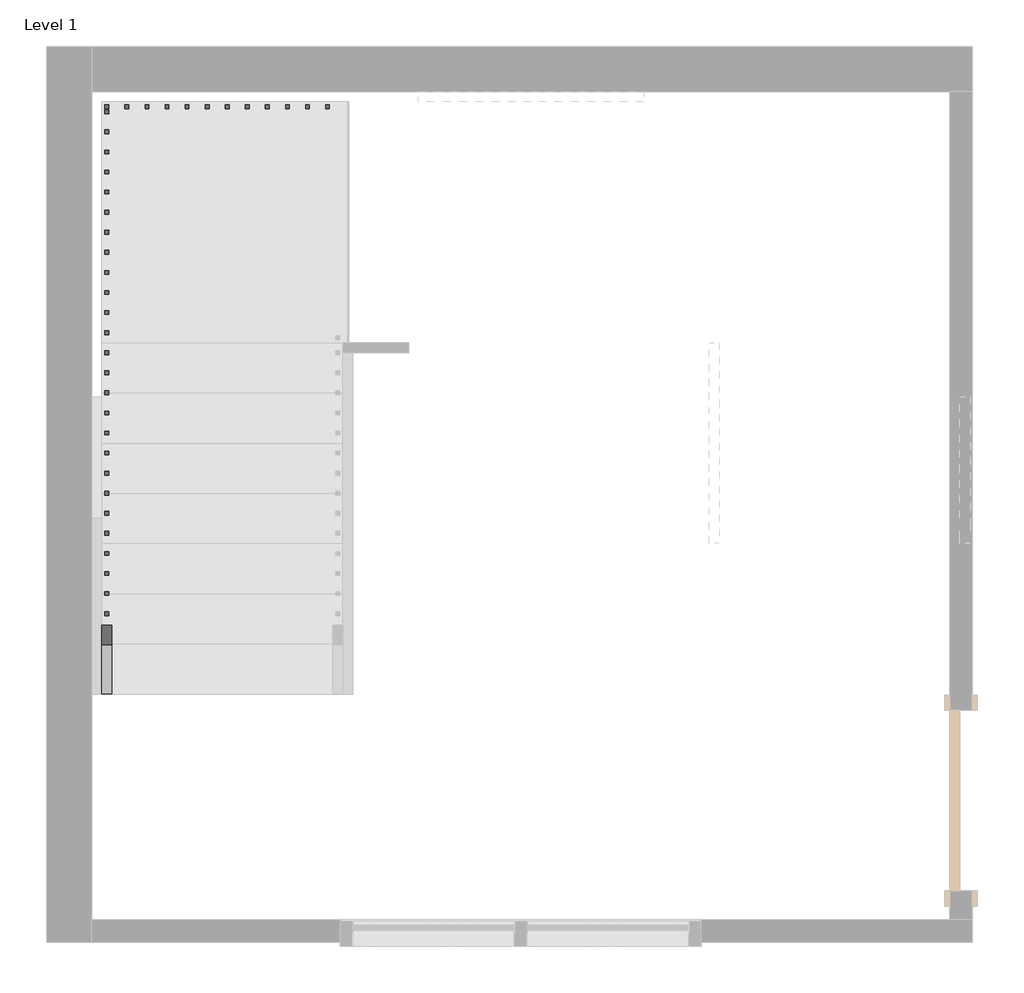
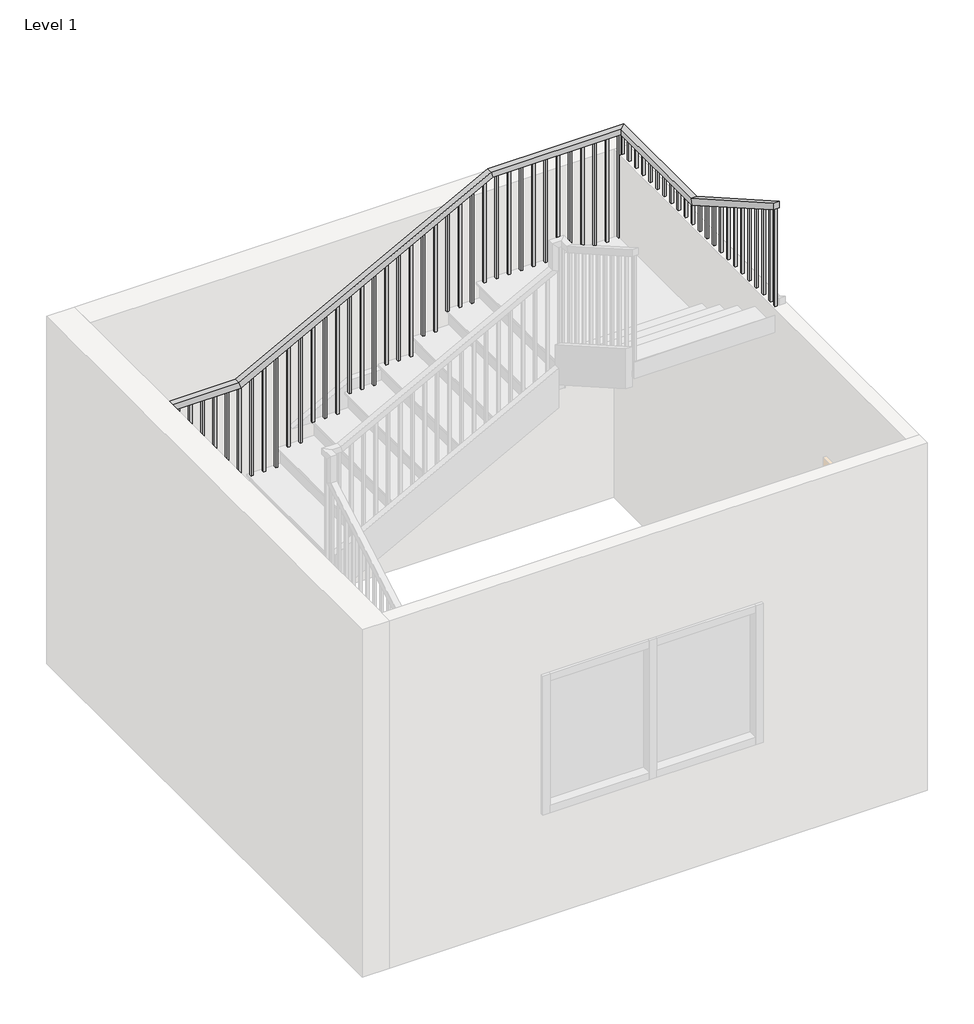
# One storey, part 5 of 9: 1 railing.
"""IFC4 building model written with IfcOpenShell, lengths in millimetres."""

from ifc_helpers import new_model, si_unit, frame, origin, place, context, project, spatial, polyline, outline, extrude, faceted_brep, element, save

model = new_model("IFC4")

# Units and contexts
model_context = context("Model", 3, world=origin())
ifc_project = project(units=[si_unit("LENGTHUNIT", "METRE", prefix="MILLI")], contexts=[model_context])

# Site, building, storey
site = spatial("IfcSite", under=ifc_project)
building = spatial("IfcBuilding", under=site)
storey = spatial("IfcBuildingStorey", under=building, Name="Level 1", Elevation=0.0)

# Railing
placement = place(None, origin())
element("IfcRailing", 1, ObjectType="Handrail - Rectangular", at=placement, inside=storey, context=model_context, shape_type="SolidModel", body=[
    faceted_brep([(-63763.8636189, 6754.3199577, 1059.5428571), (-63763.8636189, 6754.3199577, 1001.0339009), (-63713.0636189, 6754.3199577, 1001.0339009), (-63713.0636189, 6754.3199577, 1059.5428571), (-63763.8636189, 8699.113291, 2170.8533333), (-63763.8636189, 8712.6039644, 2120.0533333), (-63713.0636189, 8712.6039644, 2120.0533333), (-63713.0636189, 8699.113291, 2170.8533333), (-63763.8636189, 9751.5199577, 2170.8533333), (-63763.8636189, 9751.5199577, 2120.0533333), (-63713.0636189, 9700.7199577, 2120.0533333), (-63713.0636189, 9700.7199577, 2170.8533333), (-62638.0993332, 9751.5199577, 2170.8533333), (-62625.3993332, 9751.5199577, 2120.0533333), (-62625.3993332, 9700.7199577, 2120.0533333), (-62638.0993332, 9700.7199577, 2170.8533333), (-60546.2279046, 9751.5199577, 3286.5180952), (-60533.5279046, 9751.5199577, 3235.7180952), (-60533.5279046, 9700.7199577, 3235.7180952), (-60546.2279046, 9700.7199577, 3286.5180952), (-59420.4636189, 9751.5199577, 3286.5180952), (-59420.4636189, 9751.5199577, 3235.7180952), (-59471.2636189, 9700.7199577, 3235.7180952), (-59471.2636189, 9700.7199577, 3286.5180952), (-59420.4636189, 8699.113291, 3286.5180952), (-59420.4636189, 8685.6226176, 3235.7180952), (-59471.2636189, 8685.6226176, 3235.7180952), (-59471.2636189, 8699.113291, 3286.5180952), (-59420.4636189, 7516.3199577, 3962.4), (-59471.2636189, 7516.3199577, 3962.4), (-59471.2636189, 7516.3199577, 3903.8910438), (-59420.4636189, 7516.3199577, 3903.8910438)], [[[0, 1, 2, 3]], [[1, 0, 4, 5]], [[2, 1, 5, 6]], [[3, 2, 6, 7]], [[0, 3, 7, 4]], [[5, 4, 8, 9]], [[6, 5, 9, 10]], [[7, 6, 10, 11]], [[4, 7, 11, 8]], [[9, 8, 12, 13]], [[10, 9, 13, 14]], [[11, 10, 14, 15]], [[8, 11, 15, 12]], [[13, 12, 16, 17]], [[14, 13, 17, 18]], [[15, 14, 18, 19]], [[12, 15, 19, 16]], [[17, 16, 20, 21]], [[18, 17, 21, 22]], [[19, 18, 22, 23]], [[16, 19, 23, 20]], [[21, 20, 24, 25]], [[22, 21, 25, 26]], [[23, 22, 26, 27]], [[20, 23, 27, 24]], [[28, 29, 30, 31]], [[25, 24, 28, 31]], [[26, 25, 31, 30]], [[27, 26, 30, 29]], [[24, 27, 29, 28]]]),
    extrude(outline(polyline([(7602.0449577, 3854.9053295), (7602.0449577, 2902.8571429), (7582.9949577, 2902.8571429), (7582.9949577, 3865.7910438), (7602.0449577, 3854.9053295)])), frame((-59455.3886189, 0.0, 0.0), z_axis=(1.0, 0.0, 0.0), x_axis=(0.0, 1.0, 0.0)), (0.0, 0.0, 1.0), 19.05),
    extrude(outline(polyline([(7703.6449577, 3796.8481866), (7703.6449577, 2902.8571429), (7684.5949577, 2902.8571429), (7684.5949577, 3807.7339009), (7703.6449577, 3796.8481866)])), frame((-59455.3886189, 0.0, 0.0), z_axis=(1.0, 0.0, 0.0), x_axis=(0.0, 1.0, 0.0)), (0.0, 0.0, 1.0), 19.05),
    extrude(outline(polyline([(7805.2449577, 3738.7910438), (7805.2449577, 2757.7142857), (7786.1949577, 2757.7142857), (7786.1949577, 3749.6767581), (7805.2449577, 3738.7910438)])), frame((-59455.3886189, 0.0, 0.0), z_axis=(1.0, 0.0, 0.0), x_axis=(0.0, 1.0, 0.0)), (0.0, 0.0, 1.0), 19.05),
    extrude(outline(polyline([(7906.8449577, 3680.7339009), (7906.8449577, 2757.7142857), (7887.7949577, 2757.7142857), (7887.7949577, 3691.6196152), (7906.8449577, 3680.7339009)])), frame((-59455.3886189, 0.0, 0.0), z_axis=(1.0, 0.0, 0.0), x_axis=(0.0, 1.0, 0.0)), (0.0, 0.0, 1.0), 19.05),
    extrude(outline(polyline([(8008.4449577, 3622.6767581), (8008.4449577, 2757.7142857), (7989.3949577, 2757.7142857), (7989.3949577, 3633.5624723), (8008.4449577, 3622.6767581)])), frame((-59455.3886189, 0.0, 0.0), z_axis=(1.0, 0.0, 0.0), x_axis=(0.0, 1.0, 0.0)), (0.0, 0.0, 1.0), 19.05),
    extrude(outline(polyline([(8110.0449577, 3564.6196152), (8110.0449577, 2612.5714286), (8090.9949577, 2612.5714286), (8090.9949577, 3575.5053295), (8110.0449577, 3564.6196152)])), frame((-59455.3886189, 0.0, 0.0), z_axis=(1.0, 0.0, 0.0), x_axis=(0.0, 1.0, 0.0)), (0.0, 0.0, 1.0), 19.05),
    extrude(outline(polyline([(8211.6449577, 3506.5624723), (8211.6449577, 2612.5714286), (8192.5949577, 2612.5714286), (8192.5949577, 3517.4481866), (8211.6449577, 3506.5624723)])), frame((-59455.3886189, 0.0, 0.0), z_axis=(1.0, 0.0, 0.0), x_axis=(0.0, 1.0, 0.0)), (0.0, 0.0, 1.0), 19.05),
    extrude(outline(polyline([(8313.2449577, 3448.5053295), (8313.2449577, 2467.4285714), (8294.1949577, 2467.4285714), (8294.1949577, 3459.3910438), (8313.2449577, 3448.5053295)])), frame((-59455.3886189, 0.0, 0.0), z_axis=(1.0, 0.0, 0.0), x_axis=(0.0, 1.0, 0.0)), (0.0, 0.0, 1.0), 19.05),
    extrude(outline(polyline([(8414.8449577, 3390.4481866), (8414.8449577, 2467.4285714), (8395.7949577, 2467.4285714), (8395.7949577, 3401.3339009), (8414.8449577, 3390.4481866)])), frame((-59455.3886189, 0.0, 0.0), z_axis=(1.0, 0.0, 0.0), x_axis=(0.0, 1.0, 0.0)), (0.0, 0.0, 1.0), 19.05),
    extrude(outline(polyline([(8516.4449577, 3332.3910438), (8516.4449577, 2467.4285714), (8497.3949577, 2467.4285714), (8497.3949577, 3343.2767581), (8516.4449577, 3332.3910438)])), frame((-59455.3886189, 0.0, 0.0), z_axis=(1.0, 0.0, 0.0), x_axis=(0.0, 1.0, 0.0)), (0.0, 0.0, 1.0), 19.05),
    extrude(outline(polyline([(8618.0449577, 3274.3339009), (8618.0449577, 2322.2857143), (8598.9949577, 2322.2857143), (8598.9949577, 3285.2196152), (8618.0449577, 3274.3339009)])), frame((-59455.3886189, 0.0, 0.0), z_axis=(1.0, 0.0, 0.0), x_axis=(0.0, 1.0, 0.0)), (0.0, 0.0, 1.0), 19.05),
    extrude(outline(polyline([(-59436.3386189, 8719.6449577), (-59436.3386189, 8700.5949577), (-59455.3886189, 8700.5949577), (-59455.3886189, 8719.6449577), (-59436.3386189, 8719.6449577)])), frame((0.0, 0.0, 2322.2857143), z_axis=(0.0, 0.0, 1.0), x_axis=(1.0, 0.0, 0.0)), (0.0, 0.0, 1.0), 913.432381),
    extrude(outline(polyline([(-59436.3386189, 8821.2449577), (-59436.3386189, 8802.1949577), (-59455.3886189, 8802.1949577), (-59455.3886189, 8821.2449577), (-59436.3386189, 8821.2449577)])), frame((0.0, 0.0, 2322.2857143), z_axis=(0.0, 0.0, 1.0), x_axis=(1.0, 0.0, 0.0)), (0.0, 0.0, 1.0), 913.432381),
    extrude(outline(polyline([(-59436.3386189, 8922.8449577), (-59436.3386189, 8903.7949577), (-59455.3886189, 8903.7949577), (-59455.3886189, 8922.8449577), (-59436.3386189, 8922.8449577)])), frame((0.0, 0.0, 2322.2857143), z_axis=(0.0, 0.0, 1.0), x_axis=(1.0, 0.0, 0.0)), (0.0, 0.0, 1.0), 913.432381),
    extrude(outline(polyline([(-59436.3386189, 9024.4449577), (-59436.3386189, 9005.3949577), (-59455.3886189, 9005.3949577), (-59455.3886189, 9024.4449577), (-59436.3386189, 9024.4449577)])), frame((0.0, 0.0, 2322.2857143), z_axis=(0.0, 0.0, 1.0), x_axis=(1.0, 0.0, 0.0)), (0.0, 0.0, 1.0), 913.432381),
    extrude(outline(polyline([(-59436.3386189, 9126.0449577), (-59436.3386189, 9106.9949577), (-59455.3886189, 9106.9949577), (-59455.3886189, 9126.0449577), (-59436.3386189, 9126.0449577)])), frame((0.0, 0.0, 2322.2857143), z_axis=(0.0, 0.0, 1.0), x_axis=(1.0, 0.0, 0.0)), (0.0, 0.0, 1.0), 913.432381),
    extrude(outline(polyline([(-59436.3386189, 9227.6449577), (-59436.3386189, 9208.5949577), (-59455.3886189, 9208.5949577), (-59455.3886189, 9227.6449577), (-59436.3386189, 9227.6449577)])), frame((0.0, 0.0, 2322.2857143), z_axis=(0.0, 0.0, 1.0), x_axis=(1.0, 0.0, 0.0)), (0.0, 0.0, 1.0), 913.432381),
    extrude(outline(polyline([(-59436.3386189, 9329.2449577), (-59436.3386189, 9310.1949577), (-59455.3886189, 9310.1949577), (-59455.3886189, 9329.2449577), (-59436.3386189, 9329.2449577)])), frame((0.0, 0.0, 2322.2857143), z_axis=(0.0, 0.0, 1.0), x_axis=(1.0, 0.0, 0.0)), (0.0, 0.0, 1.0), 913.432381),
    extrude(outline(polyline([(-59436.3386189, 9430.8449577), (-59436.3386189, 9411.7949577), (-59455.3886189, 9411.7949577), (-59455.3886189, 9430.8449577), (-59436.3386189, 9430.8449577)])), frame((0.0, 0.0, 2322.2857143), z_axis=(0.0, 0.0, 1.0), x_axis=(1.0, 0.0, 0.0)), (0.0, 0.0, 1.0), 913.432381),
    extrude(outline(polyline([(-59436.3386189, 9532.4449577), (-59436.3386189, 9513.3949577), (-59455.3886189, 9513.3949577), (-59455.3886189, 9532.4449577), (-59436.3386189, 9532.4449577)])), frame((0.0, 0.0, 2322.2857143), z_axis=(0.0, 0.0, 1.0), x_axis=(1.0, 0.0, 0.0)), (0.0, 0.0, 1.0), 913.432381),
    extrude(outline(polyline([(-59436.3386189, 9634.0449577), (-59436.3386189, 9614.9949577), (-59455.3886189, 9614.9949577), (-59455.3886189, 9634.0449577), (-59436.3386189, 9634.0449577)])), frame((0.0, 0.0, 2322.2857143), z_axis=(0.0, 0.0, 1.0), x_axis=(1.0, 0.0, 0.0)), (0.0, 0.0, 1.0), 913.432381),
    extrude(outline(polyline([(-59480.7886189, 9735.6449577), (-59461.7386189, 9735.6449577), (-59461.7386189, 9716.5949577), (-59480.7886189, 9716.5949577), (-59480.7886189, 9735.6449577)])), frame((0.0, 0.0, 2322.2857143), z_axis=(0.0, 0.0, 1.0), x_axis=(1.0, 0.0, 0.0)), (0.0, 0.0, 1.0), 913.432381),
    extrude(outline(polyline([(-59582.3886189, 9735.6449577), (-59563.3386189, 9735.6449577), (-59563.3386189, 9716.5949577), (-59582.3886189, 9716.5949577), (-59582.3886189, 9735.6449577)])), frame((0.0, 0.0, 2322.2857143), z_axis=(0.0, 0.0, 1.0), x_axis=(1.0, 0.0, 0.0)), (0.0, 0.0, 1.0), 913.432381),
    extrude(outline(polyline([(-59683.9886189, 9735.6449577), (-59664.9386189, 9735.6449577), (-59664.9386189, 9716.5949577), (-59683.9886189, 9716.5949577), (-59683.9886189, 9735.6449577)])), frame((0.0, 0.0, 2322.2857143), z_axis=(0.0, 0.0, 1.0), x_axis=(1.0, 0.0, 0.0)), (0.0, 0.0, 1.0), 913.432381),
    extrude(outline(polyline([(-59785.5886189, 9735.6449577), (-59766.5386189, 9735.6449577), (-59766.5386189, 9716.5949577), (-59785.5886189, 9716.5949577), (-59785.5886189, 9735.6449577)])), frame((0.0, 0.0, 2322.2857143), z_axis=(0.0, 0.0, 1.0), x_axis=(1.0, 0.0, 0.0)), (0.0, 0.0, 1.0), 913.432381),
    extrude(outline(polyline([(-59887.1886189, 9735.6449577), (-59868.1386189, 9735.6449577), (-59868.1386189, 9716.5949577), (-59887.1886189, 9716.5949577), (-59887.1886189, 9735.6449577)])), frame((0.0, 0.0, 2322.2857143), z_axis=(0.0, 0.0, 1.0), x_axis=(1.0, 0.0, 0.0)), (0.0, 0.0, 1.0), 913.432381),
    extrude(outline(polyline([(-59988.7886189, 9735.6449577), (-59969.7386189, 9735.6449577), (-59969.7386189, 9716.5949577), (-59988.7886189, 9716.5949577), (-59988.7886189, 9735.6449577)])), frame((0.0, 0.0, 2322.2857143), z_axis=(0.0, 0.0, 1.0), x_axis=(1.0, 0.0, 0.0)), (0.0, 0.0, 1.0), 913.432381),
    extrude(outline(polyline([(-60090.3886189, 9735.6449577), (-60071.3386189, 9735.6449577), (-60071.3386189, 9716.5949577), (-60090.3886189, 9716.5949577), (-60090.3886189, 9735.6449577)])), frame((0.0, 0.0, 2322.2857143), z_axis=(0.0, 0.0, 1.0), x_axis=(1.0, 0.0, 0.0)), (0.0, 0.0, 1.0), 913.432381),
    extrude(outline(polyline([(-60191.9886189, 9735.6449577), (-60172.9386189, 9735.6449577), (-60172.9386189, 9716.5949577), (-60191.9886189, 9716.5949577), (-60191.9886189, 9735.6449577)])), frame((0.0, 0.0, 2322.2857143), z_axis=(0.0, 0.0, 1.0), x_axis=(1.0, 0.0, 0.0)), (0.0, 0.0, 1.0), 913.432381),
    extrude(outline(polyline([(-60293.5886189, 9735.6449577), (-60274.5386189, 9735.6449577), (-60274.5386189, 9716.5949577), (-60293.5886189, 9716.5949577), (-60293.5886189, 9735.6449577)])), frame((0.0, 0.0, 2322.2857143), z_axis=(0.0, 0.0, 1.0), x_axis=(1.0, 0.0, 0.0)), (0.0, 0.0, 1.0), 913.432381),
    extrude(outline(polyline([(-60395.1886189, 9735.6449577), (-60376.1386189, 9735.6449577), (-60376.1386189, 9716.5949577), (-60395.1886189, 9716.5949577), (-60395.1886189, 9735.6449577)])), frame((0.0, 0.0, 2322.2857143), z_axis=(0.0, 0.0, 1.0), x_axis=(1.0, 0.0, 0.0)), (0.0, 0.0, 1.0), 913.432381),
    extrude(outline(polyline([(-60496.7886189, 9735.6449577), (-60477.7386189, 9735.6449577), (-60477.7386189, 9716.5949577), (-60496.7886189, 9716.5949577), (-60496.7886189, 9735.6449577)])), frame((0.0, 0.0, 2322.2857143), z_axis=(0.0, 0.0, 1.0), x_axis=(1.0, 0.0, 0.0)), (0.0, 0.0, 1.0), 913.432381),
    extrude(outline(polyline([(3201.1257143, -60598.3886189), (2322.2857143, -60598.3886189), (2322.2857143, -60579.3386189), (3211.2857143, -60579.3386189), (3201.1257143, -60598.3886189)])), frame((0.0, 9716.5949577, 0.0), z_axis=(0.0, 1.0, 0.0), x_axis=(0.0, 0.0, 1.0)), (0.0, 0.0, 1.0), 19.05),
    extrude(outline(polyline([(3146.9390476, -60699.9886189), (2177.1428571, -60699.9886189), (2177.1428571, -60680.9386189), (3157.0990476, -60680.9386189), (3146.9390476, -60699.9886189)])), frame((0.0, 9716.5949577, 0.0), z_axis=(0.0, 1.0, 0.0), x_axis=(0.0, 0.0, 1.0)), (0.0, 0.0, 1.0), 19.05),
    extrude(outline(polyline([(3092.752381, -60801.5886189), (2177.1428571, -60801.5886189), (2177.1428571, -60782.5386189), (3102.912381, -60782.5386189), (3092.752381, -60801.5886189)])), frame((0.0, 9716.5949577, 0.0), z_axis=(0.0, 1.0, 0.0), x_axis=(0.0, 0.0, 1.0)), (0.0, 0.0, 1.0), 19.05),
    extrude(outline(polyline([(3038.5657143, -60903.1886189), (2177.1428571, -60903.1886189), (2177.1428571, -60884.1386189), (3048.7257143, -60884.1386189), (3038.5657143, -60903.1886189)])), frame((0.0, 9716.5949577, 0.0), z_axis=(0.0, 1.0, 0.0), x_axis=(0.0, 0.0, 1.0)), (0.0, 0.0, 1.0), 19.05),
    extrude(outline(polyline([(2984.3790476, -61004.7886189), (2032.0, -61004.7886189), (2032.0, -60985.7386189), (2994.5390476, -60985.7386189), (2984.3790476, -61004.7886189)])), frame((0.0, 9716.5949577, 0.0), z_axis=(0.0, 1.0, 0.0), x_axis=(0.0, 0.0, 1.0)), (0.0, 0.0, 1.0), 19.05),
    extrude(outline(polyline([(2930.192381, -61106.3886189), (2032.0, -61106.3886189), (2032.0, -61087.3386189), (2940.352381, -61087.3386189), (2930.192381, -61106.3886189)])), frame((0.0, 9716.5949577, 0.0), z_axis=(0.0, 1.0, 0.0), x_axis=(0.0, 0.0, 1.0)), (0.0, 0.0, 1.0), 19.05),
    extrude(outline(polyline([(2876.0057143, -61207.9886189), (1886.8571429, -61207.9886189), (1886.8571429, -61188.9386189), (2886.1657143, -61188.9386189), (2876.0057143, -61207.9886189)])), frame((0.0, 9716.5949577, 0.0), z_axis=(0.0, 1.0, 0.0), x_axis=(0.0, 0.0, 1.0)), (0.0, 0.0, 1.0), 19.05),
    extrude(outline(polyline([(2821.8190476, -61309.5886189), (1886.8571429, -61309.5886189), (1886.8571429, -61290.5386189), (2831.9790476, -61290.5386189), (2821.8190476, -61309.5886189)])), frame((0.0, 9716.5949577, 0.0), z_axis=(0.0, 1.0, 0.0), x_axis=(0.0, 0.0, 1.0)), (0.0, 0.0, 1.0), 19.05),
    extrude(outline(polyline([(2767.632381, -61411.1886189), (1886.8571429, -61411.1886189), (1886.8571429, -61392.1386189), (2777.792381, -61392.1386189), (2767.632381, -61411.1886189)])), frame((0.0, 9716.5949577, 0.0), z_axis=(0.0, 1.0, 0.0), x_axis=(0.0, 0.0, 1.0)), (0.0, 0.0, 1.0), 19.05),
    extrude(outline(polyline([(2713.4457143, -61512.7886189), (1741.7142857, -61512.7886189), (1741.7142857, -61493.7386189), (2723.6057143, -61493.7386189), (2713.4457143, -61512.7886189)])), frame((0.0, 9716.5949577, 0.0), z_axis=(0.0, 1.0, 0.0), x_axis=(0.0, 0.0, 1.0)), (0.0, 0.0, 1.0), 19.05),
    extrude(outline(polyline([(2659.2590476, -61614.3886189), (1741.7142857, -61614.3886189), (1741.7142857, -61595.3386189), (2669.4190476, -61595.3386189), (2659.2590476, -61614.3886189)])), frame((0.0, 9716.5949577, 0.0), z_axis=(0.0, 1.0, 0.0), x_axis=(0.0, 0.0, 1.0)), (0.0, 0.0, 1.0), 19.05),
    extrude(outline(polyline([(2605.072381, -61715.9886189), (1741.7142857, -61715.9886189), (1741.7142857, -61696.9386189), (2615.232381, -61696.9386189), (2605.072381, -61715.9886189)])), frame((0.0, 9716.5949577, 0.0), z_axis=(0.0, 1.0, 0.0), x_axis=(0.0, 0.0, 1.0)), (0.0, 0.0, 1.0), 19.05),
    extrude(outline(polyline([(2550.8857143, -61817.5886189), (1596.5714286, -61817.5886189), (1596.5714286, -61798.5386189), (2561.0457143, -61798.5386189), (2550.8857143, -61817.5886189)])), frame((0.0, 9716.5949577, 0.0), z_axis=(0.0, 1.0, 0.0), x_axis=(0.0, 0.0, 1.0)), (0.0, 0.0, 1.0), 19.05),
    extrude(outline(polyline([(2496.6990476, -61919.1886189), (1596.5714286, -61919.1886189), (1596.5714286, -61900.1386189), (2506.8590476, -61900.1386189), (2496.6990476, -61919.1886189)])), frame((0.0, 9716.5949577, 0.0), z_axis=(0.0, 1.0, 0.0), x_axis=(0.0, 0.0, 1.0)), (0.0, 0.0, 1.0), 19.05),
    extrude(outline(polyline([(2442.512381, -62020.7886189), (1596.5714286, -62020.7886189), (1596.5714286, -62001.7386189), (2452.672381, -62001.7386189), (2442.512381, -62020.7886189)])), frame((0.0, 9716.5949577, 0.0), z_axis=(0.0, 1.0, 0.0), x_axis=(0.0, 0.0, 1.0)), (0.0, 0.0, 1.0), 19.05),
    extrude(outline(polyline([(2388.3257143, -62122.3886189), (1451.4285714, -62122.3886189), (1451.4285714, -62103.3386189), (2398.4857143, -62103.3386189), (2388.3257143, -62122.3886189)])), frame((0.0, 9716.5949577, 0.0), z_axis=(0.0, 1.0, 0.0), x_axis=(0.0, 0.0, 1.0)), (0.0, 0.0, 1.0), 19.05),
    extrude(outline(polyline([(2334.1390476, -62223.9886189), (1451.4285714, -62223.9886189), (1451.4285714, -62204.9386189), (2344.2990476, -62204.9386189), (2334.1390476, -62223.9886189)])), frame((0.0, 9716.5949577, 0.0), z_axis=(0.0, 1.0, 0.0), x_axis=(0.0, 0.0, 1.0)), (0.0, 0.0, 1.0), 19.05),
    extrude(outline(polyline([(2279.952381, -62325.5886189), (1306.2857143, -62325.5886189), (1306.2857143, -62306.5386189), (2290.112381, -62306.5386189), (2279.952381, -62325.5886189)])), frame((0.0, 9716.5949577, 0.0), z_axis=(0.0, 1.0, 0.0), x_axis=(0.0, 0.0, 1.0)), (0.0, 0.0, 1.0), 19.05),
    extrude(outline(polyline([(2225.7657143, -62427.1886189), (1306.2857143, -62427.1886189), (1306.2857143, -62408.1386189), (2235.9257143, -62408.1386189), (2225.7657143, -62427.1886189)])), frame((0.0, 9716.5949577, 0.0), z_axis=(0.0, 1.0, 0.0), x_axis=(0.0, 0.0, 1.0)), (0.0, 0.0, 1.0), 19.05),
    extrude(outline(polyline([(2171.5790476, -62528.7886189), (1306.2857143, -62528.7886189), (1306.2857143, -62509.7386189), (2181.7390476, -62509.7386189), (2171.5790476, -62528.7886189)])), frame((0.0, 9716.5949577, 0.0), z_axis=(0.0, 1.0, 0.0), x_axis=(0.0, 0.0, 1.0)), (0.0, 0.0, 1.0), 19.05),
    extrude(outline(polyline([(2117.392381, -62630.3886189), (1161.1428571, -62630.3886189), (1161.1428571, -62611.3386189), (2127.552381, -62611.3386189), (2117.392381, -62630.3886189)])), frame((0.0, 9716.5949577, 0.0), z_axis=(0.0, 1.0, 0.0), x_axis=(0.0, 0.0, 1.0)), (0.0, 0.0, 1.0), 19.05),
    extrude(outline(polyline([(-62731.9886189, 9735.6449577), (-62712.9386189, 9735.6449577), (-62712.9386189, 9716.5949577), (-62731.9886189, 9716.5949577), (-62731.9886189, 9735.6449577)])), frame((0.0, 0.0, 1161.1428571), z_axis=(0.0, 0.0, 1.0), x_axis=(1.0, 0.0, 0.0)), (0.0, 0.0, 1.0), 958.9104762),
    extrude(outline(polyline([(-62833.5886189, 9735.6449577), (-62814.5386189, 9735.6449577), (-62814.5386189, 9716.5949577), (-62833.5886189, 9716.5949577), (-62833.5886189, 9735.6449577)])), frame((0.0, 0.0, 1161.1428571), z_axis=(0.0, 0.0, 1.0), x_axis=(1.0, 0.0, 0.0)), (0.0, 0.0, 1.0), 958.9104762),
    extrude(outline(polyline([(-62935.1886189, 9735.6449577), (-62916.1386189, 9735.6449577), (-62916.1386189, 9716.5949577), (-62935.1886189, 9716.5949577), (-62935.1886189, 9735.6449577)])), frame((0.0, 0.0, 1161.1428571), z_axis=(0.0, 0.0, 1.0), x_axis=(1.0, 0.0, 0.0)), (0.0, 0.0, 1.0), 958.9104762),
    extrude(outline(polyline([(-63036.7886189, 9735.6449577), (-63017.7386189, 9735.6449577), (-63017.7386189, 9716.5949577), (-63036.7886189, 9716.5949577), (-63036.7886189, 9735.6449577)])), frame((0.0, 0.0, 1161.1428571), z_axis=(0.0, 0.0, 1.0), x_axis=(1.0, 0.0, 0.0)), (0.0, 0.0, 1.0), 958.9104762),
    extrude(outline(polyline([(-63138.3886189, 9735.6449577), (-63119.3386189, 9735.6449577), (-63119.3386189, 9716.5949577), (-63138.3886189, 9716.5949577), (-63138.3886189, 9735.6449577)])), frame((0.0, 0.0, 1161.1428571), z_axis=(0.0, 0.0, 1.0), x_axis=(1.0, 0.0, 0.0)), (0.0, 0.0, 1.0), 958.9104762),
    extrude(outline(polyline([(-63239.9886189, 9735.6449577), (-63220.9386189, 9735.6449577), (-63220.9386189, 9716.5949577), (-63239.9886189, 9716.5949577), (-63239.9886189, 9735.6449577)])), frame((0.0, 0.0, 1161.1428571), z_axis=(0.0, 0.0, 1.0), x_axis=(1.0, 0.0, 0.0)), (0.0, 0.0, 1.0), 958.9104762),
    extrude(outline(polyline([(-63341.5886189, 9735.6449577), (-63322.5386189, 9735.6449577), (-63322.5386189, 9716.5949577), (-63341.5886189, 9716.5949577), (-63341.5886189, 9735.6449577)])), frame((0.0, 0.0, 1161.1428571), z_axis=(0.0, 0.0, 1.0), x_axis=(1.0, 0.0, 0.0)), (0.0, 0.0, 1.0), 958.9104762),
    extrude(outline(polyline([(-63443.1886189, 9735.6449577), (-63424.1386189, 9735.6449577), (-63424.1386189, 9716.5949577), (-63443.1886189, 9716.5949577), (-63443.1886189, 9735.6449577)])), frame((0.0, 0.0, 1161.1428571), z_axis=(0.0, 0.0, 1.0), x_axis=(1.0, 0.0, 0.0)), (0.0, 0.0, 1.0), 958.9104762),
    extrude(outline(polyline([(-63544.7886189, 9735.6449577), (-63525.7386189, 9735.6449577), (-63525.7386189, 9716.5949577), (-63544.7886189, 9716.5949577), (-63544.7886189, 9735.6449577)])), frame((0.0, 0.0, 1161.1428571), z_axis=(0.0, 0.0, 1.0), x_axis=(1.0, 0.0, 0.0)), (0.0, 0.0, 1.0), 958.9104762),
    extrude(outline(polyline([(-63646.3886189, 9735.6449577), (-63627.3386189, 9735.6449577), (-63627.3386189, 9716.5949577), (-63646.3886189, 9716.5949577), (-63646.3886189, 9735.6449577)])), frame((0.0, 0.0, 1161.1428571), z_axis=(0.0, 0.0, 1.0), x_axis=(1.0, 0.0, 0.0)), (0.0, 0.0, 1.0), 958.9104762),
    extrude(outline(polyline([(-63747.9886189, 9691.1949577), (-63747.9886189, 9710.2449577), (-63728.9386189, 9710.2449577), (-63728.9386189, 9691.1949577), (-63747.9886189, 9691.1949577)])), frame((0.0, 0.0, 1161.1428571), z_axis=(0.0, 0.0, 1.0), x_axis=(1.0, 0.0, 0.0)), (0.0, 0.0, 1.0), 958.9104762),
    extrude(outline(polyline([(-63747.9886189, 9589.5949577), (-63747.9886189, 9608.6449577), (-63728.9386189, 9608.6449577), (-63728.9386189, 9589.5949577), (-63747.9886189, 9589.5949577)])), frame((0.0, 0.0, 1161.1428571), z_axis=(0.0, 0.0, 1.0), x_axis=(1.0, 0.0, 0.0)), (0.0, 0.0, 1.0), 958.9104762),
    extrude(outline(polyline([(-63747.9886189, 9487.9949577), (-63747.9886189, 9507.0449577), (-63728.9386189, 9507.0449577), (-63728.9386189, 9487.9949577), (-63747.9886189, 9487.9949577)])), frame((0.0, 0.0, 1161.1428571), z_axis=(0.0, 0.0, 1.0), x_axis=(1.0, 0.0, 0.0)), (0.0, 0.0, 1.0), 958.9104762),
    extrude(outline(polyline([(-63747.9886189, 9386.3949577), (-63747.9886189, 9405.4449577), (-63728.9386189, 9405.4449577), (-63728.9386189, 9386.3949577), (-63747.9886189, 9386.3949577)])), frame((0.0, 0.0, 1161.1428571), z_axis=(0.0, 0.0, 1.0), x_axis=(1.0, 0.0, 0.0)), (0.0, 0.0, 1.0), 958.9104762),
    extrude(outline(polyline([(-63747.9886189, 9284.7949577), (-63747.9886189, 9303.8449577), (-63728.9386189, 9303.8449577), (-63728.9386189, 9284.7949577), (-63747.9886189, 9284.7949577)])), frame((0.0, 0.0, 1161.1428571), z_axis=(0.0, 0.0, 1.0), x_axis=(1.0, 0.0, 0.0)), (0.0, 0.0, 1.0), 958.9104762),
    extrude(outline(polyline([(-63747.9886189, 9183.1949577), (-63747.9886189, 9202.2449577), (-63728.9386189, 9202.2449577), (-63728.9386189, 9183.1949577), (-63747.9886189, 9183.1949577)])), frame((0.0, 0.0, 1161.1428571), z_axis=(0.0, 0.0, 1.0), x_axis=(1.0, 0.0, 0.0)), (0.0, 0.0, 1.0), 958.9104762),
    extrude(outline(polyline([(-63747.9886189, 9081.5949577), (-63747.9886189, 9100.6449577), (-63728.9386189, 9100.6449577), (-63728.9386189, 9081.5949577), (-63747.9886189, 9081.5949577)])), frame((0.0, 0.0, 1161.1428571), z_axis=(0.0, 0.0, 1.0), x_axis=(1.0, 0.0, 0.0)), (0.0, 0.0, 1.0), 958.9104762),
    extrude(outline(polyline([(-63747.9886189, 8979.9949577), (-63747.9886189, 8999.0449577), (-63728.9386189, 8999.0449577), (-63728.9386189, 8979.9949577), (-63747.9886189, 8979.9949577)])), frame((0.0, 0.0, 1161.1428571), z_axis=(0.0, 0.0, 1.0), x_axis=(1.0, 0.0, 0.0)), (0.0, 0.0, 1.0), 958.9104762),
    extrude(outline(polyline([(-63747.9886189, 8878.3949577), (-63747.9886189, 8897.4449577), (-63728.9386189, 8897.4449577), (-63728.9386189, 8878.3949577), (-63747.9886189, 8878.3949577)])), frame((0.0, 0.0, 1161.1428571), z_axis=(0.0, 0.0, 1.0), x_axis=(1.0, 0.0, 0.0)), (0.0, 0.0, 1.0), 958.9104762),
    extrude(outline(polyline([(-63747.9886189, 8776.7949577), (-63747.9886189, 8795.8449577), (-63728.9386189, 8795.8449577), (-63728.9386189, 8776.7949577), (-63747.9886189, 8776.7949577)])), frame((0.0, 0.0, 1161.1428571), z_axis=(0.0, 0.0, 1.0), x_axis=(1.0, 0.0, 0.0)), (0.0, 0.0, 1.0), 958.9104762),
    extrude(outline(polyline([(8694.2449577, 2109.5624723), (8694.2449577, 1161.1428571), (8675.1949577, 1161.1428571), (8675.1949577, 2098.6767581), (8694.2449577, 2109.5624723)])), frame((-63747.9886189, 0.0, 0.0), z_axis=(1.0, 0.0, 0.0), x_axis=(0.0, 1.0, 0.0)), (0.0, 0.0, 1.0), 19.05),
    extrude(outline(polyline([(8592.6449577, 2051.5053295), (8592.6449577, 1161.1428571), (8573.5949577, 1161.1428571), (8573.5949577, 2040.6196152), (8592.6449577, 2051.5053295)])), frame((-63747.9886189, 0.0, 0.0), z_axis=(1.0, 0.0, 0.0), x_axis=(0.0, 1.0, 0.0)), (0.0, 0.0, 1.0), 19.05),
    extrude(outline(polyline([(8491.0449577, 1993.4481866), (8491.0449577, 1016.0), (8471.9949577, 1016.0), (8471.9949577, 1982.5624723), (8491.0449577, 1993.4481866)])), frame((-63747.9886189, 0.0, 0.0), z_axis=(1.0, 0.0, 0.0), x_axis=(0.0, 1.0, 0.0)), (0.0, 0.0, 1.0), 19.05),
    extrude(outline(polyline([(8389.4449577, 1935.3910438), (8389.4449577, 1016.0), (8370.3949577, 1016.0), (8370.3949577, 1924.5053295), (8389.4449577, 1935.3910438)])), frame((-63747.9886189, 0.0, 0.0), z_axis=(1.0, 0.0, 0.0), x_axis=(0.0, 1.0, 0.0)), (0.0, 0.0, 1.0), 19.05),
    extrude(outline(polyline([(8287.8449577, 1877.3339009), (8287.8449577, 1016.0), (8268.7949577, 1016.0), (8268.7949577, 1866.4481866), (8287.8449577, 1877.3339009)])), frame((-63747.9886189, 0.0, 0.0), z_axis=(1.0, 0.0, 0.0), x_axis=(0.0, 1.0, 0.0)), (0.0, 0.0, 1.0), 19.05),
    extrude(outline(polyline([(8186.2449577, 1819.2767581), (8186.2449577, 870.8571429), (8167.1949577, 870.8571429), (8167.1949577, 1808.3910438), (8186.2449577, 1819.2767581)])), frame((-63747.9886189, 0.0, 0.0), z_axis=(1.0, 0.0, 0.0), x_axis=(0.0, 1.0, 0.0)), (0.0, 0.0, 1.0), 19.05),
    extrude(outline(polyline([(8084.6449577, 1761.2196152), (8084.6449577, 870.8571429), (8065.5949577, 870.8571429), (8065.5949577, 1750.3339009), (8084.6449577, 1761.2196152)])), frame((-63747.9886189, 0.0, 0.0), z_axis=(1.0, 0.0, 0.0), x_axis=(0.0, 1.0, 0.0)), (0.0, 0.0, 1.0), 19.05),
    extrude(outline(polyline([(7983.0449577, 1703.1624723), (7983.0449577, 725.7142857), (7963.9949577, 725.7142857), (7963.9949577, 1692.2767581), (7983.0449577, 1703.1624723)])), frame((-63747.9886189, 0.0, 0.0), z_axis=(1.0, 0.0, 0.0), x_axis=(0.0, 1.0, 0.0)), (0.0, 0.0, 1.0), 19.05),
    extrude(outline(polyline([(7881.4449577, 1645.1053295), (7881.4449577, 725.7142857), (7862.3949577, 725.7142857), (7862.3949577, 1634.2196152), (7881.4449577, 1645.1053295)])), frame((-63747.9886189, 0.0, 0.0), z_axis=(1.0, 0.0, 0.0), x_axis=(0.0, 1.0, 0.0)), (0.0, 0.0, 1.0), 19.05),
    extrude(outline(polyline([(7779.8449577, 1587.0481866), (7779.8449577, 725.7142857), (7760.7949577, 725.7142857), (7760.7949577, 1576.1624723), (7779.8449577, 1587.0481866)])), frame((-63747.9886189, 0.0, 0.0), z_axis=(1.0, 0.0, 0.0), x_axis=(0.0, 1.0, 0.0)), (0.0, 0.0, 1.0), 19.05),
    extrude(outline(polyline([(7678.2449577, 1528.9910438), (7678.2449577, 580.5714286), (7659.1949577, 580.5714286), (7659.1949577, 1518.1053295), (7678.2449577, 1528.9910438)])), frame((-63747.9886189, 0.0, 0.0), z_axis=(1.0, 0.0, 0.0), x_axis=(0.0, 1.0, 0.0)), (0.0, 0.0, 1.0), 19.05),
    extrude(outline(polyline([(7576.6449577, 1470.9339009), (7576.6449577, 580.5714286), (7557.5949577, 580.5714286), (7557.5949577, 1460.0481866), (7576.6449577, 1470.9339009)])), frame((-63747.9886189, 0.0, 0.0), z_axis=(1.0, 0.0, 0.0), x_axis=(0.0, 1.0, 0.0)), (0.0, 0.0, 1.0), 19.05),
    extrude(outline(polyline([(7475.0449577, 1412.8767581), (7475.0449577, 435.4285714), (7455.9949577, 435.4285714), (7455.9949577, 1401.9910438), (7475.0449577, 1412.8767581)])), frame((-63747.9886189, 0.0, 0.0), z_axis=(1.0, 0.0, 0.0), x_axis=(0.0, 1.0, 0.0)), (0.0, 0.0, 1.0), 19.05),
    extrude(outline(polyline([(7373.4449577, 1354.8196152), (7373.4449577, 435.4285714), (7354.3949577, 435.4285714), (7354.3949577, 1343.9339009), (7373.4449577, 1354.8196152)])), frame((-63747.9886189, 0.0, 0.0), z_axis=(1.0, 0.0, 0.0), x_axis=(0.0, 1.0, 0.0)), (0.0, 0.0, 1.0), 19.05),
    extrude(outline(polyline([(7271.8449577, 1296.7624723), (7271.8449577, 435.4285714), (7252.7949577, 435.4285714), (7252.7949577, 1285.8767581), (7271.8449577, 1296.7624723)])), frame((-63747.9886189, 0.0, 0.0), z_axis=(1.0, 0.0, 0.0), x_axis=(0.0, 1.0, 0.0)), (0.0, 0.0, 1.0), 19.05),
    extrude(outline(polyline([(7170.2449577, 1238.7053295), (7170.2449577, 290.2857143), (7151.1949577, 290.2857143), (7151.1949577, 1227.8196152), (7170.2449577, 1238.7053295)])), frame((-63747.9886189, 0.0, 0.0), z_axis=(1.0, 0.0, 0.0), x_axis=(0.0, 1.0, 0.0)), (0.0, 0.0, 1.0), 19.05),
    extrude(outline(polyline([(7068.6449577, 1180.6481866), (7068.6449577, 290.2857143), (7049.5949577, 290.2857143), (7049.5949577, 1169.7624723), (7068.6449577, 1180.6481866)])), frame((-63747.9886189, 0.0, 0.0), z_axis=(1.0, 0.0, 0.0), x_axis=(0.0, 1.0, 0.0)), (0.0, 0.0, 1.0), 19.05),
    extrude(outline(polyline([(6967.0449577, 1122.5910438), (6967.0449577, 145.1428571), (6947.9949577, 145.1428571), (6947.9949577, 1111.7053295), (6967.0449577, 1122.5910438)])), frame((-63747.9886189, 0.0, 0.0), z_axis=(1.0, 0.0, 0.0), x_axis=(0.0, 1.0, 0.0)), (0.0, 0.0, 1.0), 19.05),
    extrude(outline(polyline([(6865.4449577, 1064.5339009), (6865.4449577, 145.1428571), (6846.3949577, 145.1428571), (6846.3949577, 1053.6481866), (6865.4449577, 1064.5339009)])), frame((-63747.9886189, 0.0, 0.0), z_axis=(1.0, 0.0, 0.0), x_axis=(0.0, 1.0, 0.0)), (0.0, 0.0, 1.0), 19.05),
    extrude(outline(polyline([(-59455.3886189, 9735.6449577), (-59436.3386189, 9735.6449577), (-59436.3386189, 9716.5949577), (-59455.3886189, 9716.5949577), (-59455.3886189, 9735.6449577)])), frame((0.0, 0.0, 2322.2857143), z_axis=(0.0, 0.0, 1.0), x_axis=(1.0, 0.0, 0.0)), (0.0, 0.0, 1.0), 913.432381),
    extrude(outline(polyline([(-63747.9886189, 9716.5949577), (-63747.9886189, 9735.6449577), (-63728.9386189, 9735.6449577), (-63728.9386189, 9716.5949577), (-63747.9886189, 9716.5949577)])), frame((0.0, 0.0, 1161.1428571), z_axis=(0.0, 0.0, 1.0), x_axis=(1.0, 0.0, 0.0)), (0.0, 0.0, 1.0), 958.9104762),
    extrude(outline(polyline([(7535.3699577, 3893.0053295), (7535.3699577, 2902.8571429), (7516.3199577, 2902.8571429), (7516.3199577, 3903.8910438), (7535.3699577, 3893.0053295)])), frame((-59455.3886189, 0.0, 0.0), z_axis=(1.0, 0.0, 0.0), x_axis=(0.0, 1.0, 0.0)), (0.0, 0.0, 1.0), 19.05),
    extrude(outline(polyline([(6773.3699577, 1011.9196152), (6773.3699577, 145.1428571), (6754.3199577, 145.1428571), (6754.3199577, 1001.0339009), (6773.3699577, 1011.9196152)])), frame((-63747.9886189, 0.0, 0.0), z_axis=(1.0, 0.0, 0.0), x_axis=(0.0, 1.0, 0.0)), (0.0, 0.0, 1.0), 19.05),
])

save(model, "model.ifc")

# Revit data of these elements
# Type "Handrail - Rectangular"
#   Assembly Code = "C2010400"
#   built-in parameter 1008612 = 0.0416667 (stored number, unit not read)
#   built-in parameter 1008611 = 0.0416667 (stored number, unit not read)
#   built-in parameter 1008609 = 0.333333 (stored number, unit not read)
#   built-in parameter 1008604 = 0.166667 (stored number, unit not read)
#   built-in parameter 1008603 = 0.166667 (stored number, unit not read)
#   Railing Height = 3' - 0"
#   built-in parameter 1008630 = 2
#   built-in parameter 1008610 = 2
#   built-in parameter 1008618 = Baluster - Square : 3/4"
# Element 1 (IfcRailing, "Handrail - Rectangular")
#   Phase Created = New Construction
